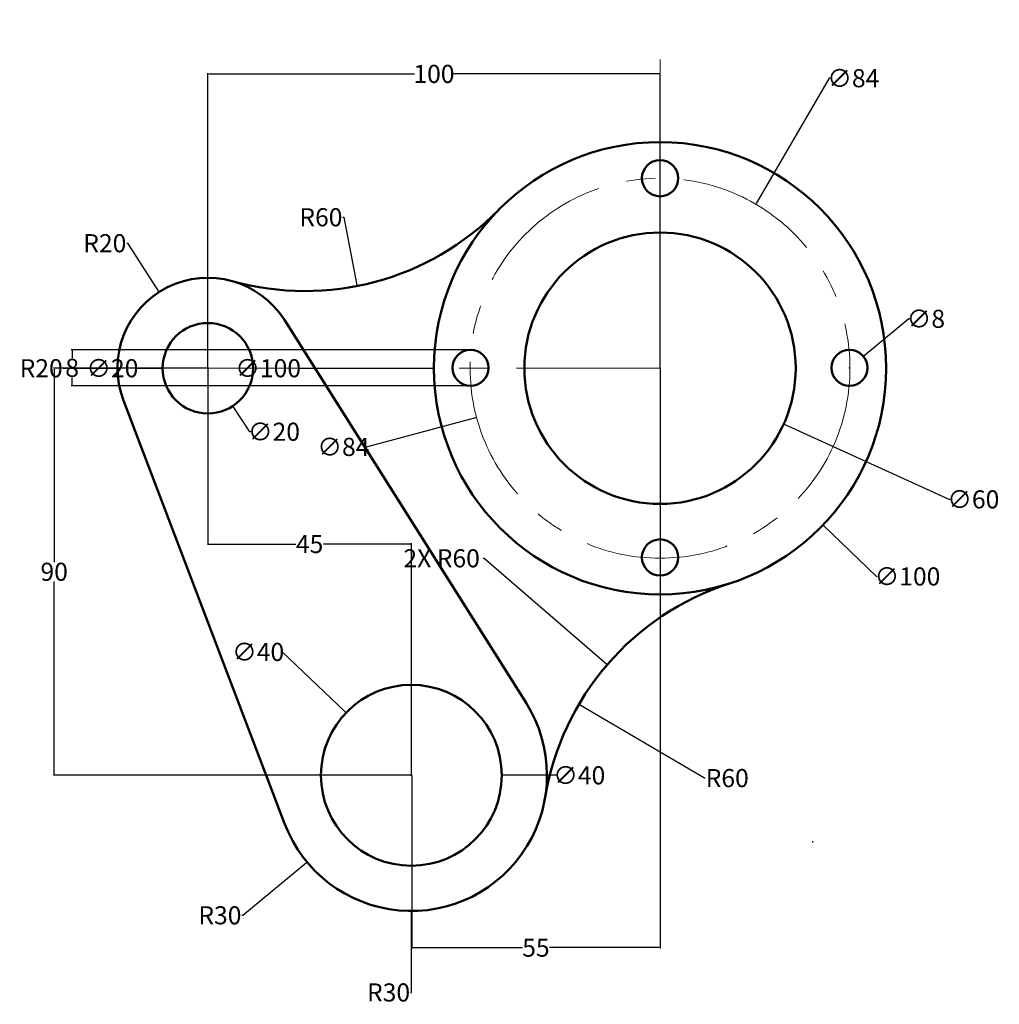
# Model space of a CAD drawing. Units: inches. Extents: x 237 to 454, y 104 to 322.
import ezdxf

# ---------------------------------------------------------------- set-up
doc = ezdxf.new("R2010")
doc.units = ezdxf.units.IN
doc.header["$MEASUREMENT"] = 0
doc.linetypes.add('CENTER', pattern=[50.8, 31.75, -6.35, 6.35, -6.35])
for name, color, linetype, lineweight in [('M-CNTR', 4, 'CENTER', 18), ('M-DIMS', 2, 'Continuous', 25), ('M-OUTL', 7, 'Continuous', 50)]:
    doc.layers.add(name, color=color, linetype=linetype, lineweight=lineweight)
doc.styles.get("Standard").update_dxf_attribs({"font": 'arial.ttf'})
doc.dimstyles.get("Standard").update_dxf_attribs({"dimtxt": 4, "dimasz": 0.18, "dimexe": 0.18, "dimexo": 0.0625, "dimgap": 0.09, "dimtad": 0, "dimtih": 1, "dimtoh": 1, "dimdec": 0, "dimzin": 0, "dimdsep": 46, "dimtxsty": 'Standard', "dimcen": 0.09, "dimadec": 0, "dimazin": 0, "dimtfac": 1, "dimtdec": 0, "dimtofl": 0, "dimtmove": 0, "dimatfit": 3, "dimfxl": 1, "dimtolj": 1, "dimtzin": 0, "dimarcsym": 0})

# ---------------------------------------------------------------- blocks, each defined once
blk = doc.blocks.new('*D1')
at = {"layer": 'Defpoints', "color": 0, "transparency": 16777216}
for p in [(378.73, 310), (278.73, 244.93), (378.73, 244.93)]:
    blk.add_point(p, dxfattribs=at)
at = {"layer": 'M-DIMS', "color": 0, "lineweight": -2, "transparency": 16777216}
for p, q in [((278.73, 244.99), (278.73, 310.18)), ((278.91, 310), (324.42, 310)), ((378.55, 310), (333.05, 310)), ((378.73, 244.99), (378.73, 310.18))]:
    blk.add_line(p, q, dxfattribs=at)
at = {"layer": 'M-DIMS', "color": 0, "transparency": 16777216}
for points in [[(278.91, 310.03), (278.91, 309.97), (278.73, 310)], [(378.55, 310.03), (378.55, 309.97), (378.73, 310)]]:
    blk.add_solid(points, dxfattribs=at)
at = {"layer": 'M-DIMS', "color": 0, "transparency": 16777216, "insert": (328.73, 310), "char_height": 4, "attachment_point": 5}
blk.add_mtext('\\A1;100', dxfattribs=at)
blk = doc.blocks.new('*D2')
at = {"layer": 'Defpoints', "color": 0, "transparency": 16777216}
for p in [(323.73, 154.93), (300.64, 135.78)]:
    blk.add_point(p, dxfattribs=at)
at = {"layer": 'M-DIMS', "color": 0, "lineweight": -2, "transparency": 16777216}
for p, q in [((323.64, 154.93), (323.82, 154.93)), ((323.73, 154.84), (323.73, 155.02)), ((286.43, 123.98), (300.51, 135.66)), ((286.25, 123.98), (286.43, 123.98))]:
    blk.add_line(p, q, dxfattribs=at)
at = {"layer": 'M-DIMS', "color": 0, "transparency": 16777216}
blk.add_solid([(300.49, 135.68), (300.53, 135.64), (300.64, 135.78)], dxfattribs=at)
at = {"layer": 'M-DIMS', "color": 0, "transparency": 16777216, "insert": (281.39, 123.98), "char_height": 4, "attachment_point": 5}
blk.add_mtext('\\A1;R30', dxfattribs=at)
blk = doc.blocks.new('*D3')
at = {"layer": 'Defpoints', "color": 0, "transparency": 16777216}
for p in [(309.27, 168.74), (338.2, 141.12)]:
    blk.add_point(p, dxfattribs=at)
at = {"layer": 'M-DIMS', "color": 0, "lineweight": -2, "transparency": 16777216}
for p, q in [((294.97, 182.21), (295.15, 182.21)), ((295.15, 182.21), (309.14, 168.86)), ((323.64, 154.93), (323.82, 154.93)), ((323.73, 154.84), (323.73, 155.02))]:
    blk.add_line(p, q, dxfattribs=at)
at = {"layer": 'M-DIMS', "color": 0, "transparency": 16777216}
blk.add_solid([(309.16, 168.88), (309.12, 168.84), (309.27, 168.74)], dxfattribs=at)
at = {"layer": 'M-DIMS', "color": 0, "transparency": 16777216, "insert": (289.85, 182.21), "char_height": 4, "attachment_point": 5}
blk.add_mtext('\\A1;∅40', dxfattribs=at)
blk = doc.blocks.new('*D4')
at = {"layer": 'Defpoints', "color": 0, "transparency": 16777216}
for p in [(278.73, 244.93), (323.73, 206.07), (323.73, 154.84)]:
    blk.add_point(p, dxfattribs=at)
at = {"layer": 'M-DIMS', "color": 0, "lineweight": -2, "transparency": 16777216}
for p, q in [((278.73, 244.87), (278.73, 205.89)), ((278.91, 206.07), (298.18, 206.07)), ((323.55, 206.07), (304.28, 206.07)), ((323.73, 154.9), (323.73, 206.25))]:
    blk.add_line(p, q, dxfattribs=at)
at = {"layer": 'M-DIMS', "color": 0, "transparency": 16777216}
for points in [[(278.91, 206.1), (278.91, 206.04), (278.73, 206.07)], [(323.55, 206.1), (323.55, 206.04), (323.73, 206.07)]]:
    blk.add_solid(points, dxfattribs=at)
at = {"layer": 'M-DIMS', "color": 0, "transparency": 16777216, "insert": (301.23, 206.07), "char_height": 4, "attachment_point": 5}
blk.add_mtext('\\A1;45', dxfattribs=at)
blk = doc.blocks.new('*D5')
at = {"layer": 'Defpoints', "color": 0, "transparency": 16777216}
for p in [(278.73, 244.93), (244.74, 154.93), (323.82, 154.93)]:
    blk.add_point(p, dxfattribs=at)
at = {"layer": 'M-DIMS', "color": 0, "lineweight": -2, "transparency": 16777216}
for p, q in [((278.67, 244.93), (244.56, 244.93)), ((244.74, 244.75), (244.74, 202.06)), ((244.74, 155.11), (244.74, 197.8)), ((323.76, 154.93), (244.56, 154.93))]:
    blk.add_line(p, q, dxfattribs=at)
at = {"layer": 'M-DIMS', "color": 0, "transparency": 16777216}
for points in [[(244.71, 244.75), (244.77, 244.75), (244.74, 244.93)], [(244.71, 155.11), (244.77, 155.11), (244.74, 154.93)]]:
    blk.add_solid(points, dxfattribs=at)
at = {"layer": 'M-DIMS', "color": 0, "transparency": 16777216, "insert": (244.74, 199.93), "char_height": 4, "attachment_point": 5}
blk.add_mtext('\\A1;90', dxfattribs=at)
blk = doc.blocks.new('*D6')
at = {"layer": 'Defpoints', "color": 0, "transparency": 16777216}
for p in [(378.73, 244.93), (323.82, 154.93), (378.73, 116.83)]:
    blk.add_point(p, dxfattribs=at)
at = {"layer": 'M-DIMS', "color": 0, "lineweight": -2, "transparency": 16777216}
for p, q in [((378.73, 244.87), (378.73, 116.65)), ((323.82, 154.87), (323.82, 116.65)), ((324, 116.83), (348.31, 116.83)), ((378.55, 116.83), (354.25, 116.83))]:
    blk.add_line(p, q, dxfattribs=at)
at = {"layer": 'M-DIMS', "color": 0, "transparency": 16777216}
for points in [[(324, 116.86), (324, 116.8), (323.82, 116.83)], [(378.55, 116.86), (378.55, 116.8), (378.73, 116.83)]]:
    blk.add_solid(points, dxfattribs=at)
at = {"layer": 'M-DIMS', "color": 0, "transparency": 16777216, "insert": (351.28, 116.83), "char_height": 4, "attachment_point": 5}
blk.add_mtext('\\A1;55', dxfattribs=at)
blk = doc.blocks.new('*D7')
at = {"layer": 'Defpoints', "color": 0, "transparency": 16777216}
for p in [(300.23, 321.99), (311.74, 263.1)]:
    blk.add_point(p, dxfattribs=at)
at = {"layer": 'M-DIMS', "color": 0, "lineweight": -2, "transparency": 16777216}
for p, q in [((308.59, 278.31), (308.77, 278.31)), ((308.77, 278.31), (311.71, 263.28))]:
    blk.add_line(p, q, dxfattribs=at)
at = {"layer": 'M-DIMS', "color": 0, "transparency": 16777216}
blk.add_solid([(311.74, 263.28), (311.68, 263.27), (311.74, 263.1)], dxfattribs=at)
at = {"layer": 'M-DIMS', "color": 0, "transparency": 16777216, "insert": (303.73, 278.31), "char_height": 4, "attachment_point": 5}
blk.add_mtext('\\A1;R60', dxfattribs=at)
blk = doc.blocks.new('*D8')
at = {"layer": 'Defpoints', "color": 0, "transparency": 16777216}
for p in [(360.78, 170.61), (412.53, 140.25)]:
    blk.add_point(p, dxfattribs=at)
at = {"layer": 'M-DIMS', "color": 0, "lineweight": -2, "transparency": 16777216}
for p, q in [((388.55, 154.32), (360.93, 170.52)), ((388.73, 154.32), (388.55, 154.32))]:
    blk.add_line(p, q, dxfattribs=at)
at = {"layer": 'M-DIMS', "color": 0, "transparency": 16777216}
blk.add_solid([(360.95, 170.55), (360.92, 170.49), (360.78, 170.61)], dxfattribs=at)
at = {"layer": 'M-DIMS', "color": 0, "transparency": 16777216, "insert": (393.59, 154.32), "char_height": 4, "attachment_point": 5}
blk.add_mtext('\\A1;R60', dxfattribs=at)
blk = doc.blocks.new('*D9')
at = {"layer": 'Defpoints', "color": 0, "transparency": 16777216}
for p in [(342.7, 279.59), (414.77, 210.27)]:
    blk.add_point(p, dxfattribs=at)
at = {"layer": 'M-DIMS', "color": 0, "lineweight": -2, "transparency": 16777216}
for p, q in [((378.64, 244.93), (378.82, 244.93)), ((378.73, 244.84), (378.73, 245.02)), ((426.59, 198.9), (414.9, 210.15)), ((426.77, 198.9), (426.59, 198.9))]:
    blk.add_line(p, q, dxfattribs=at)
at = {"layer": 'M-DIMS', "color": 0, "transparency": 16777216}
blk.add_solid([(414.92, 210.17), (414.88, 210.12), (414.77, 210.27)], dxfattribs=at)
at = {"layer": 'M-DIMS', "color": 0, "transparency": 16777216, "insert": (433.45, 198.9), "char_height": 4, "attachment_point": 5}
blk.add_mtext('\\A1;∅100', dxfattribs=at)
blk = doc.blocks.new('*D10')
at = {"layer": 'Defpoints', "color": 0, "transparency": 16777216}
for p in [(399.91, 281.2), (357.56, 208.66)]:
    blk.add_point(p, dxfattribs=at)
at = {"layer": 'M-DIMS', "color": 0, "lineweight": -2, "transparency": 16777216}
for p, q in [((416.17, 309.05), (400, 281.36)), ((416.35, 309.05), (416.17, 309.05)), ((378.64, 244.93), (378.82, 244.93)), ((378.73, 244.84), (378.73, 245.02))]:
    blk.add_line(p, q, dxfattribs=at)
at = {"layer": 'M-DIMS', "color": 0, "transparency": 16777216}
blk.add_solid([(399.98, 281.37), (400.03, 281.34), (399.91, 281.2)], dxfattribs=at)
at = {"layer": 'M-DIMS', "color": 0, "transparency": 16777216, "insert": (421.47, 309.05), "char_height": 4, "attachment_point": 5}
blk.add_mtext('\\A1;∅84', dxfattribs=at)
blk = doc.blocks.new('*D11')
at = {"layer": 'Defpoints', "color": 0, "transparency": 16777216}
for p in [(351.41, 257.31), (406.06, 232.55)]:
    blk.add_point(p, dxfattribs=at)
at = {"layer": 'M-DIMS', "color": 0, "lineweight": -2, "transparency": 16777216}
for p, q in [((378.64, 244.93), (378.82, 244.93)), ((378.73, 244.84), (378.73, 245.02)), ((442.7, 215.94), (406.22, 232.47)), ((442.88, 215.94), (442.7, 215.94))]:
    blk.add_line(p, q, dxfattribs=at)
at = {"layer": 'M-DIMS', "color": 0, "transparency": 16777216}
blk.add_solid([(406.24, 232.5), (406.21, 232.45), (406.06, 232.55)], dxfattribs=at)
at = {"layer": 'M-DIMS', "color": 0, "transparency": 16777216, "insert": (448.01, 215.94), "char_height": 4, "attachment_point": 5}
blk.add_mtext('\\A1;∅60', dxfattribs=at)
blk = doc.blocks.new('*U12')
blk.add_circle((0, 0), 4)
blk = doc.blocks.new('*U13')
at = {"layer": 'M-OUTL', "color": 0, "linetype": 'ByBlock', "lineweight": -2, "transparency": 16777216}
blk.add_blockref('*U12', (378.73, 286.93), dxfattribs=at)
for p, rotation in [((336.82, 245.02), 90), ((420.64, 245.02), 270.0000000000001), ((378.73, 203.11), 180)]:
    blk.add_blockref('*U12', p, dxfattribs=dict(at, rotation=rotation))
blk = doc.blocks.new('*D14')
at = {"layer": 'Defpoints', "color": 0, "transparency": 16777216}
for p in [(267.92, 261.76), (278.73, 244.93)]:
    blk.add_point(p, dxfattribs=at)
at = {"layer": 'M-DIMS', "color": 0, "lineweight": -2, "transparency": 16777216}
for p, q in [((260.8, 272.57), (260.98, 272.57)), ((260.98, 272.57), (267.83, 261.91)), ((278.64, 244.93), (278.82, 244.93)), ((278.73, 244.84), (278.73, 245.02))]:
    blk.add_line(p, q, dxfattribs=at)
at = {"layer": 'M-DIMS', "color": 0, "transparency": 16777216}
blk.add_solid([(267.85, 261.92), (267.8, 261.89), (267.92, 261.76)], dxfattribs=at)
at = {"layer": 'M-DIMS', "color": 0, "transparency": 16777216, "insert": (255.94, 272.57), "char_height": 4, "attachment_point": 5}
blk.add_mtext('\\A1;R20', dxfattribs=at)
blk = doc.blocks.new('*D15')
at = {"layer": 'Defpoints', "color": 0, "transparency": 16777216}
for p in [(273.21, 253.27), (284.26, 236.59)]:
    blk.add_point(p, dxfattribs=at)
at = {"layer": 'M-DIMS', "color": 0, "lineweight": -2, "transparency": 16777216}
for p, q in [((278.64, 244.93), (278.82, 244.93)), ((278.73, 244.84), (278.73, 245.02)), ((288.04, 230.89), (284.36, 236.44)), ((288.22, 230.89), (288.04, 230.89))]:
    blk.add_line(p, q, dxfattribs=at)
at = {"layer": 'M-DIMS', "color": 0, "transparency": 16777216}
blk.add_solid([(284.38, 236.46), (284.33, 236.43), (284.26, 236.59)], dxfattribs=at)
at = {"layer": 'M-DIMS', "color": 0, "transparency": 16777216, "insert": (293.34, 230.89), "char_height": 4, "attachment_point": 5}
blk.add_mtext('\\A1;∅20', dxfattribs=at)
blk = doc.blocks.new('*D16')
at = {"layer": 'Defpoints', "color": 0, "transparency": 16777216}
for p in [(423.73, 247.57), (417.56, 242.47)]:
    blk.add_point(p, dxfattribs=at)
at = {"layer": 'M-DIMS', "color": 0, "lineweight": -2, "transparency": 16777216}
for p, q in [((433.76, 255.86), (423.87, 247.68)), ((433.94, 255.86), (433.76, 255.86)), ((420.55, 245.02), (420.73, 245.02)), ((420.64, 244.93), (420.64, 245.11))]:
    blk.add_line(p, q, dxfattribs=at)
at = {"layer": 'M-DIMS', "color": 0, "transparency": 16777216}
blk.add_solid([(423.85, 247.71), (423.89, 247.66), (423.73, 247.57)], dxfattribs=at)
at = {"layer": 'M-DIMS', "color": 0, "transparency": 16777216, "insert": (437.52, 255.86), "char_height": 4, "width": 6.9823, "attachment_point": 5}
blk.add_mtext('\\A1;∅8', dxfattribs=at)
blk = doc.blocks.new('*D17')
at = {"layer": 'Defpoints', "color": 0, "transparency": 16777216}
for p in [(248.71, 249.02), (336.82, 249.02), (336.82, 241.02)]:
    blk.add_point(p, dxfattribs=at)
at = {"layer": 'M-DIMS', "color": 0, "lineweight": -2, "transparency": 16777216}
for p, q in [((336.76, 249.02), (248.53, 249.02)), ((248.71, 248.84), (248.71, 247.15)), ((248.71, 241.2), (248.71, 242.89)), ((336.76, 241.02), (248.53, 241.02))]:
    blk.add_line(p, q, dxfattribs=at)
at = {"layer": 'M-DIMS', "color": 0, "transparency": 16777216}
for points in [[(248.68, 248.84), (248.74, 248.84), (248.71, 249.02)], [(248.68, 241.2), (248.74, 241.2), (248.71, 241.02)]]:
    blk.add_solid(points, dxfattribs=at)
at = {"layer": 'M-DIMS', "color": 0, "transparency": 16777216, "insert": (248.71, 245.02), "char_height": 4, "attachment_point": 5}
blk.add_mtext('\\A1;8', dxfattribs=at)
blk = doc.blocks.new('*D18')
at = {"layer": 'Defpoints', "color": 0, "transparency": 16777216}
for p in [(328.73, 244.93), (428.73, 244.93)]:
    blk.add_point(p, dxfattribs=at)
at = {"layer": 'M-DIMS', "color": 0, "lineweight": -2, "transparency": 16777216}
for p, q in [((298.73, 244.93), (328.55, 244.93)), ((378.64, 244.93), (378.82, 244.93)), ((378.73, 244.84), (378.73, 245.02))]:
    blk.add_line(p, q, dxfattribs=at)
at = {"layer": 'M-DIMS', "color": 0, "transparency": 16777216}
blk.add_solid([(328.55, 244.96), (328.55, 244.9), (328.73, 244.93)], dxfattribs=at)
at = {"layer": 'M-DIMS', "color": 0, "transparency": 16777216, "insert": (292.06, 244.93), "char_height": 4, "attachment_point": 5}
blk.add_mtext('\\A1;∅100', dxfattribs=at)
blk = doc.blocks.new('*D19')
at = {"layer": 'Defpoints', "color": 0, "transparency": 16777216}
for p in [(419.3, 255.8), (338.17, 234.06)]:
    blk.add_point(p, dxfattribs=at)
at = {"layer": 'M-DIMS', "color": 0, "lineweight": -2, "transparency": 16777216}
for p, q in [((378.64, 244.93), (378.82, 244.93)), ((378.73, 244.84), (378.73, 245.02)), ((313.82, 227.54), (337.99, 234.01))]:
    blk.add_line(p, q, dxfattribs=at)
at = {"layer": 'M-DIMS', "color": 0, "transparency": 16777216}
blk.add_solid([(337.98, 234.04), (338, 233.98), (338.17, 234.06)], dxfattribs=at)
at = {"layer": 'M-DIMS', "color": 0, "transparency": 16777216, "insert": (308.7, 227.54), "char_height": 4, "attachment_point": 5}
blk.add_mtext('\\A1;∅84', dxfattribs=at)
blk = doc.blocks.new('*D20')
at = {"layer": 'Defpoints', "color": 0, "transparency": 16777216}
for p in [(258.73, 244.93), (278.73, 244.93)]:
    blk.add_point(p, dxfattribs=at)
at = {"layer": 'M-DIMS', "color": 0, "lineweight": -2, "transparency": 16777216}
for p, q in [((246.73, 244.93), (258.55, 244.93)), ((278.64, 244.93), (278.82, 244.93)), ((278.73, 244.84), (278.73, 245.02))]:
    blk.add_line(p, q, dxfattribs=at)
at = {"layer": 'M-DIMS', "color": 0, "transparency": 16777216}
blk.add_solid([(258.55, 244.96), (258.55, 244.9), (258.73, 244.93)], dxfattribs=at)
at = {"layer": 'M-DIMS', "color": 0, "transparency": 16777216, "insert": (241.87, 244.93), "char_height": 4, "attachment_point": 5}
blk.add_mtext('\\A1;R20', dxfattribs=at)
blk = doc.blocks.new('*D21')
at = {"layer": 'Defpoints', "color": 0, "transparency": 16777216}
for p in [(268.73, 244.93), (288.73, 244.93)]:
    blk.add_point(p, dxfattribs=at)
at = {"layer": 'M-DIMS', "color": 0, "lineweight": -2, "transparency": 16777216}
for p, q in [((262.73, 244.93), (268.55, 244.93)), ((278.64, 244.93), (278.82, 244.93)), ((278.73, 244.84), (278.73, 245.02))]:
    blk.add_line(p, q, dxfattribs=at)
at = {"layer": 'M-DIMS', "color": 0, "transparency": 16777216}
blk.add_solid([(268.55, 244.96), (268.55, 244.9), (268.73, 244.93)], dxfattribs=at)
at = {"layer": 'M-DIMS', "color": 0, "transparency": 16777216, "insert": (257.61, 244.93), "char_height": 4, "attachment_point": 5}
blk.add_mtext('\\A1;∅20', dxfattribs=at)
blk = doc.blocks.new('*D22')
at = {"layer": 'Defpoints', "color": 0, "transparency": 16777216}
for p in [(367.07, 179.41), (412.53, 140.25)]:
    blk.add_point(p, dxfattribs=at)
at = {"layer": 'M-DIMS', "color": 0, "lineweight": -2, "transparency": 16777216}
for p, q in [((339.62, 202.91), (339.8, 202.91)), ((339.8, 202.91), (366.94, 179.53)), ((412.44, 140.25), (412.62, 140.25)), ((412.53, 140.16), (412.53, 140.34))]:
    blk.add_line(p, q, dxfattribs=at)
at = {"layer": 'M-DIMS', "color": 0, "transparency": 16777216}
blk.add_solid([(366.96, 179.55), (366.92, 179.51), (367.07, 179.41)], dxfattribs=at)
at = {"layer": 'M-DIMS', "color": 0, "transparency": 16777216, "insert": (330.43, 202.91), "char_height": 4, "attachment_point": 5}
blk.add_mtext('\\A1;2X R60', dxfattribs=at)
blk = doc.blocks.new('*D23')
at = {"layer": 'Defpoints', "color": 0, "transparency": 16777216}
for p in [(303.73, 154.93), (343.73, 154.93)]:
    blk.add_point(p, dxfattribs=at)
at = {"layer": 'M-DIMS', "color": 0, "lineweight": -2, "transparency": 16777216}
for p, q in [((323.64, 154.93), (323.82, 154.93)), ((323.73, 154.84), (323.73, 155.02)), ((355.73, 154.93), (343.91, 154.93))]:
    blk.add_line(p, q, dxfattribs=at)
at = {"layer": 'M-DIMS', "color": 0, "transparency": 16777216}
blk.add_solid([(343.91, 154.96), (343.91, 154.9), (343.73, 154.93)], dxfattribs=at)
at = {"layer": 'M-DIMS', "color": 0, "transparency": 16777216, "insert": (360.86, 154.93), "char_height": 4, "attachment_point": 5}
blk.add_mtext('\\A1;∅40', dxfattribs=at)
blk = doc.blocks.new('*D24')
at = {"layer": 'Defpoints', "color": 0, "transparency": 16777216}
for p in [(323.73, 154.93), (323.73, 124.93)]:
    blk.add_point(p, dxfattribs=at)
at = {"layer": 'M-DIMS', "color": 0, "lineweight": -2, "transparency": 16777216}
for p, q in [((323.64, 154.93), (323.82, 154.93)), ((323.73, 154.84), (323.73, 155.02)), ((323.73, 106.93), (323.73, 124.75)), ((323.55, 106.93), (323.73, 106.93))]:
    blk.add_line(p, q, dxfattribs=at)
at = {"layer": 'M-DIMS', "color": 0, "transparency": 16777216}
blk.add_solid([(323.7, 124.75), (323.76, 124.75), (323.73, 124.93)], dxfattribs=at)
at = {"layer": 'M-DIMS', "color": 0, "transparency": 16777216, "insert": (318.69, 106.93), "char_height": 4, "attachment_point": 5}
blk.add_mtext('\\A1;R30', dxfattribs=at)

msp = doc.modelspace()

# ---------------------------------------------------------------- linework, layer by layer
at = {"layer": 'M-CNTR'}
for p, q in [((378.73, 313.15), (378.73, 173.82)), ((278.73, 264.93), (278.73, 221.8)), ((298.73, 244.93), (258.73, 244.93)), ((378.73, 244.93), (328.73, 244.93))]:
    msp.add_line(p, q, dxfattribs=at)
msp.add_circle((378.73, 244.93), 42, dxfattribs=at)
at = {"layer": 'M-OUTL'}
for p, q in [((295.65, 255.61), (349.1, 170.95)), ((260.05, 237.81), (295.7, 144.25))]:
    msp.add_line(p, q, dxfattribs=at)
for centre, radius in [((378.73, 244.93), 50), ((378.73, 244.93), 30), ((278.73, 244.93), 10), ((323.73, 154.93), 20)]:
    msp.add_circle(centre, radius, dxfattribs=at)
for centre, radius, start, end in [((300.23, 321.99), 60, 254.4101, 315.5316), ((278.73, 244.93), 20, 32.2686, 200.8615), ((412.53, 140.25), 60, 107.892, 170.6124), ((323.73, 154.93), 30, 200.8615, 32.2686)]:
    msp.add_arc(centre, radius, start, end, dxfattribs=at)

# ---------------------------------------------------------------- block references
msp.add_blockref('*U13', (0, 0), dxfattribs=at)

# ---------------------------------------------------------------- dimensions: what is measured, and where the dimension line sits
at = {"layer": 'M-DIMS'}
for center, mpoint, override, picture, middle in [((300.23, 321.99), (311.74, 263.1), {"dimclrd": 0, "dimclre": 0, "dimclrt": 0}, '*D7', (303.73, 278.31)), ((278.73, 244.93), (267.92, 261.76), {"dimclrd": 0, "dimclre": 0, "dimclrt": 0}, '*D14', (255.94, 272.57)), ((278.73, 244.93), (258.73, 244.93), {"dimdec": 0, "dimlfac": 1, "dimrnd": 0, "dimzin": 0, "dimdsep": 46, "dimlunit": 2}, '*D20', (246.73, 244.93)), ((412.53, 140.25), (360.78, 170.61), {"dimclrd": 0, "dimclre": 0, "dimclrt": 0}, '*D8', (393.59, 154.32)), ((323.73, 154.93), (300.64, 135.78), {"dimclrd": 0, "dimclre": 0, "dimclrt": 0}, '*D2', (281.39, 123.98)), ((323.73, 154.93), (323.73, 124.93), {"dimdec": 0, "dimlfac": 1, "dimrnd": 0, "dimzin": 0, "dimdsep": 46, "dimlunit": 2}, '*D24', (318.69, 106.93))]:
    dim = msp.add_radius_dim(center=center, mpoint=mpoint, dimstyle='Standard', override=override, dxfattribs=at)
    dim.commit()
    dim.dimension.update_dxf_attribs({"geometry": picture, "text_midpoint": middle, "dimtype": 164})
dim = msp.add_linear_dim(base=(378.73, 310), p1=(278.73, 244.93), p2=(378.73, 244.93), dimstyle='Standard', override={"dimclrd": 0, "dimclre": 0, "dimclrt": 0}, dxfattribs=at)
dim.commit()
dim.dimension.update_dxf_attribs({"geometry": '*D1', "text_midpoint": (328.73, 310), "dimtype": 160})
for p1, p2, override, picture, middle in [((357.56, 208.66), (399.91, 281.2), {"dimclrd": 0, "dimclre": 0, "dimclrt": 0}, '*D10', (421.47, 309.05)), ((342.7, 279.59), (414.77, 210.27), {"dimclrd": 0, "dimclre": 0, "dimclrt": 0}, '*D9', (433.45, 198.9)), ((351.41, 257.31), (406.06, 232.55), {"dimclrd": 0, "dimclre": 0, "dimclrt": 0}, '*D11', (448.01, 215.94)), ((417.56, 242.47), (423.73, 247.57), {"dimclrd": 0, "dimclre": 0, "dimclrt": 0}, '*D16', (437.52, 255.86)), ((419.3, 255.8), (338.17, 234.06), {"dimdec": 0, "dimlfac": 1, "dimrnd": 0, "dimzin": 0, "dimdsep": 46, "dimlunit": 2}, '*D19', (313.82, 227.54)), ((273.21, 253.27), (284.26, 236.59), {"dimclrd": 0, "dimclre": 0, "dimclrt": 0}, '*D15', (293.34, 230.89)), ((288.73, 244.93), (268.73, 244.93), {"dimdec": 0, "dimlfac": 1, "dimrnd": 0, "dimzin": 0, "dimdsep": 46, "dimlunit": 2}, '*D21', (262.73, 244.93)), ((428.73, 244.93), (328.73, 244.93), {"dimdec": 0, "dimlfac": 1, "dimrnd": 0, "dimzin": 0, "dimdsep": 46, "dimlunit": 2}, '*D18', (298.73, 244.93)), ((338.2, 141.12), (309.27, 168.74), {"dimclrd": 0, "dimclre": 0, "dimclrt": 0}, '*D3', (289.85, 182.21)), ((303.73, 154.93), (343.73, 154.93), {"dimdec": 0, "dimlfac": 1, "dimrnd": 0, "dimzin": 0, "dimdsep": 46, "dimlunit": 2}, '*D23', (355.73, 154.93))]:
    dim = msp.add_diameter_dim_2p(p1=p1, p2=p2, dimstyle='Standard', override=override, dxfattribs=at)
    dim.commit()
    dim.dimension.update_dxf_attribs({"geometry": picture, "text_midpoint": middle, "dimtype": 163})
for base, p1, p2, override, picture, middle in [((248.71, 249.02), (336.82, 241.02), (336.82, 249.02), {"dimdec": 0, "dimlfac": 1, "dimrnd": 0, "dimzin": 0, "dimdsep": 46, "dimlunit": 2}, '*D17', (248.71, 245.02)), ((244.74, 154.93), (278.73, 244.93), (323.82, 154.93), {"dimclrd": 0, "dimclre": 0, "dimclrt": 0}, '*D5', (244.74, 199.93))]:
    dim = msp.add_linear_dim(base=base, p1=p1, p2=p2, angle=90, dimstyle='Standard', override=override, dxfattribs=at)
    dim.commit()
    dim.dimension.update_dxf_attribs({"geometry": picture, "text_midpoint": middle})
for base, p1, p2, picture, middle in [((323.73, 206.07), (278.73, 244.93), (323.73, 154.84), '*D4', (301.23, 206.07)), ((378.73, 116.83), (323.82, 154.93), (378.73, 244.93), '*D6', (351.28, 116.83))]:
    dim = msp.add_linear_dim(base=base, p1=p1, p2=p2, dimstyle='Standard', override={"dimclrd": 0, "dimclre": 0, "dimclrt": 0}, dxfattribs=at)
    dim.commit()
    dim.dimension.update_dxf_attribs({"geometry": picture, "text_midpoint": middle})
dim = msp.add_radius_dim(center=(412.53, 140.25), mpoint=(367.07, 179.41), text='2X <>', dimstyle='Standard', override={"dimdec": 0, "dimlfac": 1, "dimrnd": 0, "dimzin": 0, "dimdsep": 46, "dimlunit": 2}, dxfattribs=at)
dim.commit()
dim.dimension.update_dxf_attribs({"geometry": '*D22', "text_midpoint": (330.43, 202.91), "dimtype": 164})

doc.saveas('drawing.dxf')
